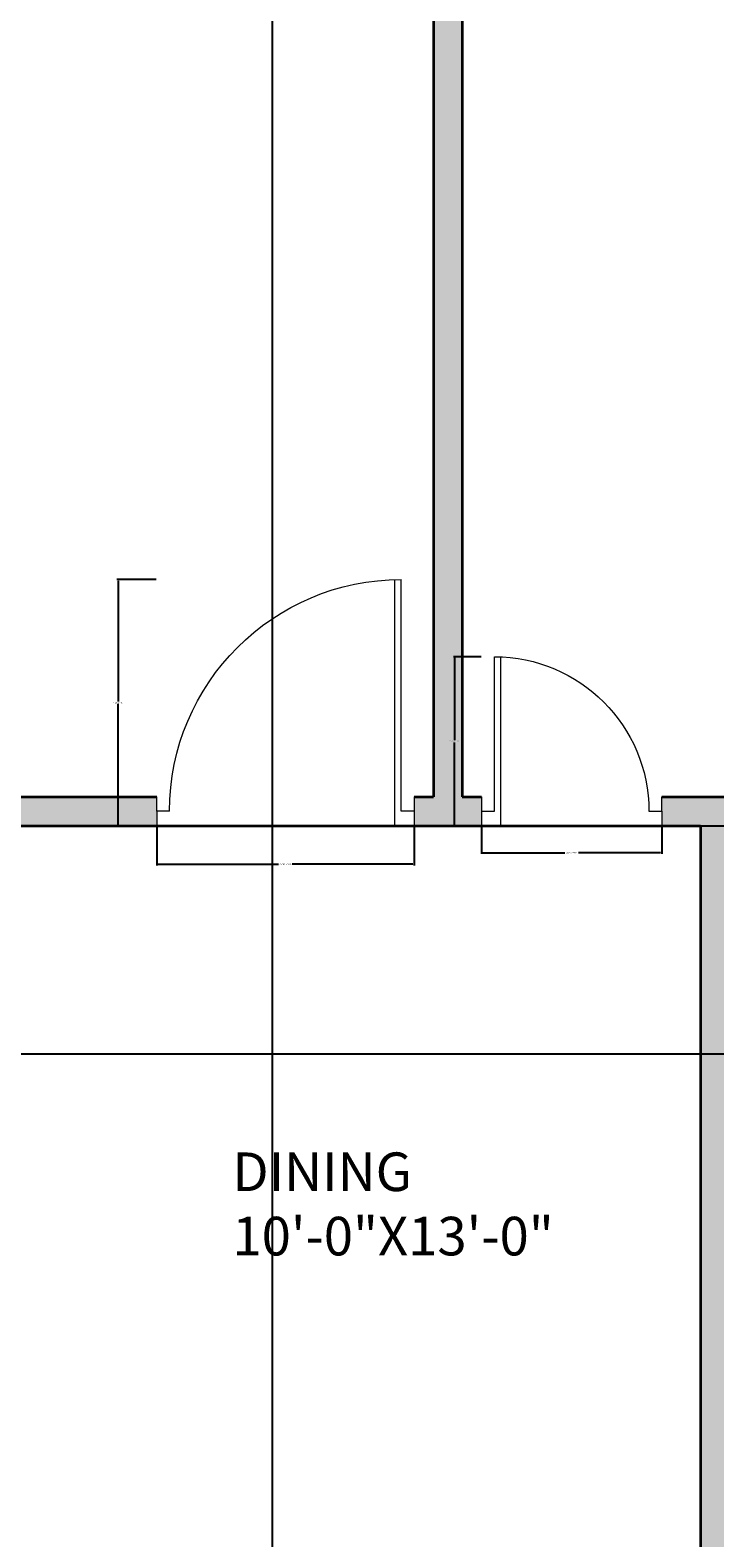
# Model space of a CAD drawing. Units: inches. Extents: x -15 to 423, y -713 to 71.
# Tile 9 of 24: x 144 to 251, y -351 to -117. Entities that reach past the tile are written whole.
import ezdxf

# ---------------------------------------------------------------- set-up
doc = ezdxf.new("R2010")
doc.units = ezdxf.units.IN
doc.header["$MEASUREMENT"] = 0
for name, color, linetype, lineweight in [('A-ANNO-DIMS', 2, 'Continuous', 18), ('A-AREA-IDEN', 7, 'Continuous', 18), ('A-DOOR', 3, 'Continuous', 18), ('A-WALL', 7, 'Continuous', 35), ('A-WALL-PATT', 8, 'Continuous', 13)]:
    doc.layers.add(name, color=color, linetype=linetype, lineweight=lineweight)
doc.styles.get("Standard").update_dxf_attribs({"font": 'arial.ttf'})
doc.dimstyles.get("Standard").update_dxf_attribs({"dimtxt": 0.18, "dimasz": 0.18, "dimexe": 0.18, "dimexo": 0.0625, "dimgap": 0.09, "dimtad": 0, "dimtih": 1, "dimtoh": 1, "dimdec": 0, "dimzin": 0, "dimdsep": 46, "dimlunit": 3, "dimtxsty": 'Standard', "dimcen": 0.09, "dimadec": 0, "dimazin": 0, "dimtfac": 1, "dimtdec": 0, "dimtofl": 0, "dimtmove": 0, "dimatfit": 3, "dimfxl": 1, "dimtolj": 1, "dimtzin": 0, "dimarcsym": 0})

# ---------------------------------------------------------------- blocks, each defined once
blk = doc.blocks.new('DOOR-24IN-JAMB4_5')
for p, q in [((25, 0), (25, 26.25)), ((26, 2.25), (26, 26.25)), ((0, 2.25), (0, 4.5)), ((28, 4.5), (28, 0)), ((2, 2.25), (0, 2.25)), ((0, 2.25), (0, 0)), ((28, 2.25), (26, 2.25))]:
    blk.add_line(p, q)
blk.add_arc((26, 2.25), 24, 90, 180)
blk = doc.blocks.new('DOOR-36IN-JAMB4_5')
for p, q in [((2, 2.25), (2, 38.25)), ((3, 0), (3, 38.25)), ((0, 4.5), (0, 0)), ((40, 2.25), (40, 4.5)), ((0, 2.25), (2, 2.25)), ((38, 2.25), (40, 2.25)), ((40, 2.25), (40, 0))]:
    blk.add_line(p, q)
blk.add_arc((2, 2.25), 36, 0, 90)
blk = doc.blocks.new('*D25')
at = {"layer": 'A-ANNO-DIMS', "color": 0, "lineweight": -2, "transparency": 16777216}
for p, q in [((214.58, -240.56), (214.58, -244.88)), ((242.58, -240.56), (242.58, -244.88)), ((214.76, -244.7), (227.53, -244.7)), ((242.4, -244.7), (229.63, -244.7))]:
    blk.add_line(p, q, dxfattribs=at)
at = {"layer": 'A-ANNO-DIMS', "color": 0, "transparency": 16777216}
for points in [[(214.76, -244.67), (214.76, -244.73), (214.58, -244.7)], [(242.4, -244.67), (242.4, -244.73), (242.58, -244.7)]]:
    blk.add_solid(points, dxfattribs=at)
at = {"layer": 'Defpoints', "color": 0, "transparency": 16777216}
for p in [(214.58, -240.5), (242.58, -240.5), (214.58, -244.7)]:
    blk.add_point(p, dxfattribs=at)
at = {"layer": 'A-ANNO-DIMS', "color": 0, "transparency": 16777216, "insert": (228.58, -244.7), "char_height": 0.18, "attachment_point": 5}
blk.add_mtext('\\A1;DOOR 2\'-4" TYP.', dxfattribs=at)
blk = doc.blocks.new('*D26')
at = {"layer": 'A-ANNO-DIMS', "color": 0, "lineweight": -2, "transparency": 16777216}
for p, q in [((214.52, -214.25), (210.2, -214.25)), ((210.38, -214.43), (210.38, -227.19)), ((210.38, -240.32), (210.38, -227.56)), ((214.52, -240.5), (210.2, -240.5))]:
    blk.add_line(p, q, dxfattribs=at)
at = {"layer": 'A-ANNO-DIMS', "color": 0, "transparency": 16777216}
for points in [[(210.35, -214.43), (210.41, -214.43), (210.38, -214.25)], [(210.35, -240.32), (210.41, -240.32), (210.38, -240.5)]]:
    blk.add_solid(points, dxfattribs=at)
at = {"layer": 'Defpoints', "color": 0, "transparency": 16777216}
for p in [(210.38, -214.25), (214.58, -214.25), (214.58, -240.5)]:
    blk.add_point(p, dxfattribs=at)
at = {"layer": 'A-ANNO-DIMS', "color": 0, "transparency": 16777216, "insert": (210.38, -227.37), "char_height": 0.18, "attachment_point": 5}
blk.add_mtext('\\A1;2\'-2 1/2" TYP.', dxfattribs=at)
blk = doc.blocks.new('*D27')
at = {"layer": 'A-ANNO-DIMS', "color": 0, "lineweight": -2, "transparency": 16777216}
for p, q in [((164.08, -240.56), (164.08, -246.68)), ((204.08, -240.56), (204.08, -246.68)), ((164.26, -246.5), (183.03, -246.5)), ((203.9, -246.5), (185.13, -246.5))]:
    blk.add_line(p, q, dxfattribs=at)
at = {"layer": 'A-ANNO-DIMS', "color": 0, "transparency": 16777216}
for points in [[(164.26, -246.47), (164.26, -246.53), (164.08, -246.5)], [(203.9, -246.47), (203.9, -246.53), (204.08, -246.5)]]:
    blk.add_solid(points, dxfattribs=at)
at = {"layer": 'Defpoints', "color": 0, "transparency": 16777216}
for p in [(164.08, -240.5), (204.08, -240.5), (164.08, -246.5)]:
    blk.add_point(p, dxfattribs=at)
at = {"layer": 'A-ANNO-DIMS', "color": 0, "transparency": 16777216, "insert": (184.08, -246.5), "char_height": 0.18, "attachment_point": 5}
blk.add_mtext('\\A1;DOOR 3\'-4" TYP.', dxfattribs=at)
blk = doc.blocks.new('*D28')
at = {"layer": 'A-ANNO-DIMS', "color": 0, "lineweight": -2, "transparency": 16777216}
for p, q in [((164.02, -202.25), (157.9, -202.25)), ((158.08, -202.43), (158.08, -221.19)), ((158.08, -240.32), (158.08, -221.56)), ((164.02, -240.5), (157.9, -240.5))]:
    blk.add_line(p, q, dxfattribs=at)
at = {"layer": 'A-ANNO-DIMS', "color": 0, "transparency": 16777216}
for points in [[(158.05, -202.43), (158.11, -202.43), (158.08, -202.25)], [(158.05, -240.32), (158.11, -240.32), (158.08, -240.5)]]:
    blk.add_solid(points, dxfattribs=at)
at = {"layer": 'Defpoints', "color": 0, "transparency": 16777216}
for p in [(158.08, -202.25), (164.08, -202.25), (164.08, -240.5)]:
    blk.add_point(p, dxfattribs=at)
at = {"layer": 'A-ANNO-DIMS', "color": 0, "transparency": 16777216, "insert": (158.08, -221.37), "char_height": 0.18, "attachment_point": 5}
blk.add_mtext('\\A1;3\'-2 1/2" TYP.', dxfattribs=at)
blk = doc.blocks.new('*D38')
at = {"layer": 'A-ANNO-DIMS', "color": 0, "lineweight": -2, "transparency": 16777216}
for p, q in [((124.14, -240.5), (422.01, -240.5)), ((421.83, -240.68), (421.83, -258.06)), ((421.83, -275.8), (421.83, -258.42)), ((124.14, -275.98), (422.01, -275.98))]:
    blk.add_line(p, q, dxfattribs=at)
at = {"layer": 'A-ANNO-DIMS', "color": 0, "transparency": 16777216}
for points in [[(421.8, -240.68), (421.86, -240.68), (421.83, -240.5)], [(421.8, -275.8), (421.86, -275.8), (421.83, -275.98)]]:
    blk.add_solid(points, dxfattribs=at)
at = {"layer": 'Defpoints', "color": 0, "transparency": 16777216}
for p in [(124.08, -240.5), (124.08, -275.98), (421.83, -275.98)]:
    blk.add_point(p, dxfattribs=at)
at = {"layer": 'A-ANNO-DIMS', "color": 0, "transparency": 16777216, "insert": (421.83, -258.24), "char_height": 0.18, "attachment_point": 5}
blk.add_mtext('\\A1;2\'-11 1/2"', dxfattribs=at)
blk = doc.blocks.new('*D42')
at = {"layer": 'A-ANNO-DIMS', "color": 0, "lineweight": -2, "transparency": 16777216}
for p, q in [((133.08, -409.94), (133.08, 57.43)), ((133.26, 57.25), (157.25, 57.25)), ((181.9, 57.25), (157.91, 57.25)), ((182.08, -409.94), (182.08, 57.43))]:
    blk.add_line(p, q, dxfattribs=at)
at = {"layer": 'A-ANNO-DIMS', "color": 0, "transparency": 16777216}
for points in [[(133.26, 57.28), (133.26, 57.22), (133.08, 57.25)], [(181.9, 57.28), (181.9, 57.22), (182.08, 57.25)]]:
    blk.add_solid(points, dxfattribs=at)
at = {"layer": 'Defpoints', "color": 0, "transparency": 16777216}
for p in [(182.08, 57.25), (133.08, -410), (182.08, -410)]:
    blk.add_point(p, dxfattribs=at)
at = {"layer": 'A-ANNO-DIMS', "color": 0, "transparency": 16777216, "insert": (157.58, 57.25), "char_height": 0.18, "attachment_point": 5}
blk.add_mtext('\\A1;4\'-1"', dxfattribs=at)

msp = doc.modelspace()

# ---------------------------------------------------------------- hatches: boundary and pattern name
at = {"layer": 'A-WALL-PATT'}
h = msp.add_hatch(color=256, dxfattribs=at)
h.dxf.hatch_style = 1
h.paths.add_polyline_path([(34.08, -349.58), (25.08, -349.58), (25.08, -431), (34.08, -431)])
h.paths.add_polyline_path([(34.08, -467), (25.08, -467), (25.08, -673), (34.08, -673)])
h.paths.add_polyline_path([(373.08, -668.5), (182.08, -668.5), (182.08, -673), (373.08, -673)])
h.paths.add_polyline_path([(253.2, -597.5), (191.08, -597.5), (191.08, -594.5), (182.08, -594.5), (182.08, -606.5), (253.2, -606.5)])
h.paths.add_polyline_path([(373.08, -597.5), (313.2, -597.5), (313.2, -606.5), (373.08, -606.5)])
h.paths.add_polyline_path([(382.08, -545.55), (373.08, -545.55), (373.08, -673), (382.08, -673)])
h.paths.add_polyline_path([(139.08, -488), (34.08, -488), (34.08, -497), (139.08, -497), (139.08, -492.5)])
h.paths.add_polyline_path([(139.08, -396.5), (128.58, -396.5), (128.58, -352.79), (124.08, -352.79), (124.08, -396.5), (34.08, -396.5), (34.08, -410), (139.08, -410), (139.08, -403.25)])
h.paths.add_polyline_path([(191.08, -396.5), (179.08, -396.5), (179.08, -410), (182.08, -410), (182.08, -488), (179.08, -488), (179.08, -497), (182.08, -497), (182.08, -501.43), (191.08, -501.43)])
h.paths.add_polyline_path([(373.08, -396.5), (253.08, -396.5), (253.08, -393.5), (248.58, -393.5), (248.58, -401), (284.58, -401), (284.58, -404), (289.08, -404), (289.08, -401), (373.08, -401)])
h.paths.add_polyline_path([(373.08, -449), (289.08, -449), (289.08, -432), (286.83, -432), (284.58, -432), (284.58, -453.5), (373.08, -453.5)])
h.paths.add_polyline_path([(382.08, -344.27), (373.08, -344.27), (373.08, -413.68), (382.08, -413.68)])
h.paths.add_polyline_path([(382.08, -437.68), (373.08, -437.68), (373.08, -485.55), (382.08, -485.55)])
h.paths.add_polyline_path([(34.08, -188.26), (25.08, -188.26), (25.08, -289.58), (34.08, -289.58)])
h.paths.add_polyline_path([(164.08, -236), (34.08, -236), (34.08, -240.5), (124.08, -240.5), (124.08, -293.12), (128.58, -293.12), (128.58, -240.5), (164.08, -240.5), (164.08, -238.25)])
h.paths.add_polyline_path([(373.08, -236), (242.58, -236), (242.58, -238.25), (242.58, -240.5), (248.58, -240.5), (248.58, -353.5), (250.83, -353.5), (253.08, -353.5), (253.08, -240.5), (373.08, -240.5)])
h.paths.add_polyline_path([(382.08, -190.86), (373.08, -190.86), (373.08, -284.27), (382.08, -284.27)])
h.paths.add_polyline_path([(211.58, -80), (253.58, -80), (253.58, -77.75), (253.58, -75.5), (153.58, -75.5), (153.58, -77.75), (153.58, -80), (207.08, -80), (207.08, -236), (204.08, -236), (204.08, -240.5), (214.58, -240.5), (214.58, -236), (211.58, -236)])
h.paths.add_polyline_path([(34.08, 8.5), (70.36, 8.5), (70.36, 17.5), (25.08, 17.5), (25.08, -128.26), (34.08, -128.26)])
h.paths.add_polyline_path([(110.58, 17.5), (94.36, 17.5), (94.36, 8.5), (110.58, 8.5)])
h.paths.add_polyline_path([(296.58, 17.5), (110.58, 17.5), (110.58, 13), (296.58, 13)])
h.paths.add_polyline_path([(110.58, 8.5), (106.08, 8.5), (106.08, -75.5), (103.08, -75.5), (103.08, -80), (113.58, -80), (113.58, -77.75), (113.58, -75.5), (110.58, -75.5)])
h.paths.add_polyline_path([(75.08, -75.5), (34.08, -75.5), (34.08, -80), (75.08, -80), (75.08, -77.75)])
h.paths.add_polyline_path([(343.09, 17.5), (296.58, 17.5), (296.58, 13), (296.58, 8.5), (343.09, 8.5)])
h.paths.add_polyline_path([(304.08, -75.5), (301.08, -75.5), (301.08, 8.5), (296.58, 8.5), (296.58, -75.5), (293.58, -75.5), (293.58, -80), (304.08, -80)])
h.paths.add_polyline_path([(382.08, 17.5), (367.09, 17.5), (367.09, 8.5), (373.08, 8.5), (373.08, -130.86), (382.08, -130.86)])
h.paths.add_polyline_path([(373.08, -75.5), (332.08, -75.5), (332.08, -77.75), (332.08, -80), (373.08, -80)])

# ---------------------------------------------------------------- linework, layer by layer
at = {"layer": 'A-WALL'}
for p, q in [((207.08, -80), (207.08, -236)), ((211.58, -80), (211.58, -236)), ((34.08, -236), (164.08, -236)), ((204.08, -236), (207.08, -236)), ((211.58, -236), (214.58, -236)), ((242.58, -236), (373.08, -236)), ((128.58, -240.5), (248.58, -240.5)), ((248.58, -240.5), (248.58, -401))]:
    msp.add_line(p, q, dxfattribs=at)

# ---------------------------------------------------------------- block references
at = {"layer": 'A-DOOR', "extrusion": (0, 0, -1), "zscale": -1}
for name, p in [('DOOR-36IN-JAMB4_5', (-204.08, -240.5)), ('DOOR-24IN-JAMB4_5', (-242.58, -240.5))]:
    msp.add_blockref(name, p, dxfattribs=at)

# ---------------------------------------------------------------- texts
at = {"layer": 'A-AREA-IDEN', "insert": (175.85, -291.29), "char_height": 6, "attachment_point": 1}
msp.add_mtext('DINING\\P10\'-0"X13\'-0"', dxfattribs=at)

# ---------------------------------------------------------------- dimensions: what is measured, and where the dimension line sits
at = {"layer": 'A-ANNO-DIMS'}
dim = msp.add_linear_dim(base=(182.08, 57.25), p1=(133.08, -410), p2=(182.08, -410), dimstyle='Standard', override={"dimdec": 1, "dimlfac": 1, "dimrnd": 0, "dimzin": 1, "dimdsep": 46, "dimlunit": 4, "dimfrac": 2}, dxfattribs=at)
dim.commit()
dim.dimension.update_dxf_attribs({"geometry": '*D42', "text_midpoint": (157.58, 57.25)})
for base, p1, p2, angle, text, picture, middle in [((158.08055573, -202.24989936), (164.08055573, -240.49989936), (164.08055573, -202.24989936), 90, '<> TYP.', '*D28', (158.08055573, -221.37489936)), ((210.38055573, -214.24989936), (214.58055573, -240.49989936), (214.58055573, -214.24989936), 90, '<> TYP.', '*D26', (210.38055573, -227.37489936)), ((164.08, -246.5), (204.08, -240.5), (164.08, -240.5), 180, 'DOOR <> TYP.', '*D27', (184.08, -246.5)), ((214.58, -244.7), (242.58, -240.5), (214.58, -240.5), 180, 'DOOR <> TYP.', '*D25', (228.58, -244.7))]:
    dim = msp.add_linear_dim(base=base, p1=p1, p2=p2, angle=angle, text=text, dimstyle='Standard', override={"dimdec": 1, "dimlfac": 1, "dimrnd": 0, "dimzin": 1, "dimdsep": 46, "dimlunit": 4, "dimfrac": 2}, dxfattribs=at)
    dim.commit()
    dim.dimension.update_dxf_attribs({"geometry": picture, "text_midpoint": middle})
dim = msp.add_linear_dim(base=(421.83, -275.98), p1=(124.08, -240.5), p2=(124.08, -275.98), angle=90, dimstyle='Standard', override={"dimdec": 1, "dimlfac": 1, "dimrnd": 0, "dimzin": 1, "dimdsep": 46, "dimlunit": 4, "dimfrac": 2}, dxfattribs=at)
dim.commit()
dim.dimension.update_dxf_attribs({"geometry": '*D38', "text_midpoint": (421.83, -258.24)})

doc.saveas('drawing.dxf')
